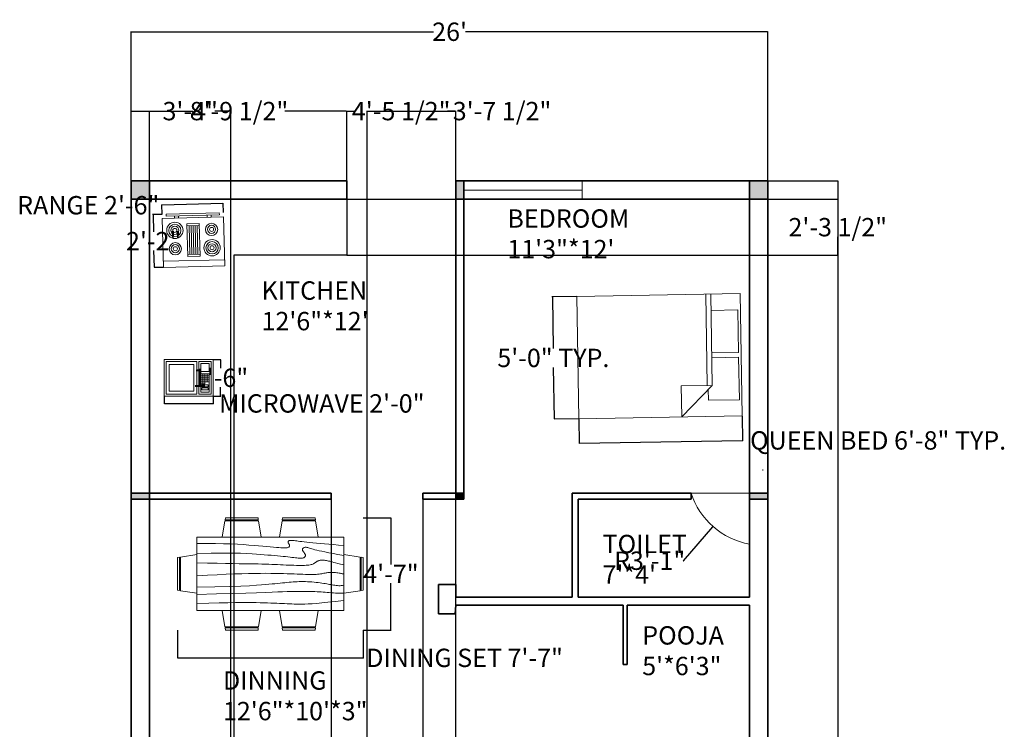
# Model space of a CAD drawing. Units: inches. Extents: x 23641 to 24129, y 27170 to 27889.
# Tile 2 of 2: x 23646 to 24129, y 27541 to 27889. Entities that reach past the tile are written whole.
import ezdxf

# ---------------------------------------------------------------- set-up
doc = ezdxf.new("R2010")
doc.units = ezdxf.units.IN
doc.header["$MEASUREMENT"] = 0
for name, color, linetype, lineweight in [('A-ANNO-DIMS', 2, 'Continuous', 18), ('A-AREA-IDEN', 7, 'Continuous', 25), ('A-DOOR', 4, 'Continuous', 18), ('A-EQPM', 9, 'Continuous', 18), ('A-FLOR-CASE', 8, 'Continuous', 25), ('A-FURN', 8, 'Continuous', 18), ('A-GLAZ', 4, 'Continuous', 18), ('A-WALL', 7, 'Continuous', 35), ('A-WALL-PATT', 7, 'Continuous', 13)]:
    doc.layers.add(name, color=color, linetype=linetype, lineweight=lineweight)
doc.styles.get("Standard").update_dxf_attribs({"font": 'arial.ttf'})
doc.dimstyles.get("Standard").update_dxf_attribs({"dimtxt": 9, "dimasz": 0.18, "dimexe": 0.18, "dimexo": 0.0625, "dimgap": 0.09, "dimtad": 0, "dimtih": 1, "dimtoh": 1, "dimdec": 0, "dimzin": 0, "dimdsep": 46, "dimlunit": 3, "dimtxsty": 'Standard', "dimcen": 0.09, "dimadec": 0, "dimazin": 0, "dimtfac": 1, "dimtdec": 0, "dimtofl": 0, "dimtmove": 0, "dimatfit": 3, "dimfxl": 1, "dimtolj": 1, "dimtzin": 0, "dimarcsym": 0})

# ---------------------------------------------------------------- blocks, each defined once
blk = doc.blocks.new('Range-Oven - 30 in top')
for p, q in [((0, -3), (30, -3)), ((12, -6), (18, -6)), ((13, -20), (13, -6)), ((14, -6), (14, -20)), ((15, -20), (15, -6)), ((16, -6), (16, -20)), ((17, -20), (17, -6)), ((6, -24), (6, -25)), ((8, -25), (8, -24)), ((18, -20), (12, -20)), ((22, -25), (22, -24)), ((24, -24), (24, -25))]:
    blk.add_line(p, q)
for points in [[(0, -24), (0, 0), (30, 0), (30, -24)], [(12, -21), (12, -5), (18, -5), (18, -21)], [(2, -26), (2, -25), (28, -25), (28, -26)]]:
    blk.add_lwpolyline(points, close=True)
for centre, radius in [((6, -9), 4), ((6, -9), 3), ((6, -9), 2), ((6, -9), 1), ((24, -9), 3), ((24, -9), 2), ((24, -9), 1), ((24, -18), 4), ((6, -18), 3), ((6, -18), 2), ((6, -18), 1), ((24, -18), 3), ((24, -18), 2), ((24, -18), 1)]:
    blk.add_circle(centre, radius)
blk = doc.blocks.new('Microwave')
for p, q in [((18, 10), (22, 10)), ((19, 7), (19, 11)), ((20, 11), (20, 7)), ((21, 7), (21, 11)), ((22, 9), (18, 9)), ((18, 8), (22, 8)), ((22, 7), (18, 7)), ((20, 6), (18, 6)), ((19, 6), (19, 7)), ((20, 7), (20, 6))]:
    blk.add_line(p, q)
for points in [[(0, 0), (0, 18), (24, 18), (24, 0)], [(1, 1), (1, 17), (16, 17), (16, 1)], [(2.5, 2.5), (2.5, 15.5), (14.5, 15.5), (14.5, 2.5)], [(17, 1), (17, 17), (23, 17), (23, 1)], [(18, 12), (18, 16), (22, 16), (22, 12)], [(18, 2), (18, 11), (22, 11), (22, 2)], [(18.5, 4.5), (18.5, 5.5), (21.5, 5.5), (21.5, 4.5)], [(18.5, 3), (18.5, 4), (21.5, 4), (21.5, 3)]]:
    blk.add_lwpolyline(points, close=True)
blk = doc.blocks.new('Dining Set - 36 x 72 in.')
for p, q in [((-22.2343, 26.00059), (-23.4847, 17.99762)), ((-22.2304, 26), (-5.7608, 26)), ((-22, 27.5), (-22.1562, 26.50042)), ((-5.8416, 26.5), (-22.1534, 26.5)), ((-22, 27.5), (-6, 27.5)), ((-5.8437, 26.49966), (-6, 27.5)), ((-4.5152, 17.99762), (-5.7655, 25.99926)), ((5.7657, 26.00059), (4.5153, 17.99762)), ((5.7696, 26), (22.2392, 26)), ((6, 27.5), (5.8438, 26.50042)), ((22.1584, 26.5), (5.8466, 26.5)), ((6, 27.5), (22, 27.5)), ((22.1563, 26.49966), (22, 27.5)), ((23.4848, 17.99762), (22.2345, 25.99926)), ((36, 18), (-36, 18)), ((-36, 18), (-36, -18)), ((36, -18), (36, 18)), ((-45.5, 8), (-44.5004, 8.15617)), ((-45.5, 8), (-45.5, -8)), ((-44.5, -8.15843), (-44.5, 8.15338)), ((-44.0006, 8.23428), (-35.9976, 9.48474)), ((-44, 8.23041), (-44, -8.23915)), ((44.0006, 8.23428), (35.9976, 9.48474)), ((44, 8.23041), (44, -8.23915)), ((44.5, -8.15843), (44.5, 8.15338)), ((45.5, 8), (44.5005, 8.15617)), ((45.5, 8), (45.5, -8)), ((-44.4997, -8.15631), (-45.5, -8)), ((-35.9976, -9.48476), (-43.9993, -8.2345)), ((35.9976, -9.48476), (43.9993, -8.2345)), ((44.4997, -8.15631), (45.5, -8)), ((-36, -18), (36, -18)), ((-22.2343, -26.0006), (-23.4847, -17.99762)), ((-4.5152, -17.99762), (-5.7655, -25.99928)), ((5.7657, -26.0006), (4.5153, -17.99762)), ((23.4848, -17.99762), (22.2345, -25.99928)), ((-22.2304, -26), (-5.7608, -26)), ((-22, -27.5), (-22.1562, -26.50044)), ((-5.8416, -26.5), (-22.1534, -26.5)), ((-22, -27.5), (-6, -27.5)), ((-5.8437, -26.49967), (-6, -27.5)), ((5.7696, -26), (22.2392, -26)), ((6, -27.5), (5.8438, -26.50044)), ((22.1584, -26.5), (5.8466, -26.5)), ((6, -27.5), (22, -27.5)), ((22.1563, -26.49967), (22, -27.5))]:
    blk.add_line(p, q)
for points in [[(-36, 15), (-31.1772, 14.97754), (-26.8079, 14.91406), (-22.8538, 14.81543), (-19.276, 14.6875), (-16.0362, 14.53613), (-13.0957, 14.36718), (-10.4159, 14.18652), (-7.9583, 14), (-5.6904, 13.81315), (-3.6035, 13.63021), (-1.6954, 13.45508), (0.0365, 13.29166), (1.5945, 13.14388), (2.9811, 13.01562), (4.1988, 12.9108), (5.25, 12.83333), (6.1393, 12.78613), (6.8802, 12.76823), (7.4883, 12.77767), (7.9792, 12.8125), (8.3685, 12.87077), (8.6719, 12.95052), (8.9049, 13.0498), (9.0833, 13.16666), (9.2205, 13.29899), (9.3216, 13.44401), (9.3895, 13.59879), (9.4271, 13.76041), (9.4373, 13.92594), (9.4232, 14.09245), (9.3875, 14.257), (9.3333, 14.41666), (9.2638, 14.56917), (9.1836, 14.71484), (9.0975, 14.85465), (9.0104, 14.98958), (8.9272, 15.1206), (8.8529, 15.2487), (8.7922, 15.37483), (8.75, 15.5), (8.7305, 15.62467), (8.7344, 15.74739), (8.7617, 15.86621), (8.8125, 15.97916), (8.8867, 16.08431), (8.9844, 16.17968), (9.1055, 16.26334), (9.25, 16.33333), (9.4189, 16.38802), (9.6172, 16.42708), (9.8506, 16.45052), (10.125, 16.45833), (10.4463, 16.45052), (10.8203, 16.42708), (11.2529, 16.38802), (11.75, 16.33333), (12.3184, 16.26318), (12.9694, 16.17838), (13.7151, 16.07991), (14.5677, 15.96875), (15.5395, 15.84586), (16.6426, 15.71224), (17.8893, 15.56884), (19.2917, 15.41666), (20.859, 15.25667), (22.5879, 15.08984), (24.4721, 14.91715), (26.5052, 14.73958), (28.6809, 14.5581), (30.9929, 14.3737), (33.4347, 14.18733), (36, 14)], [(-36, 10), (-28.9766, 10.14274), (-23.1725, 10.20442), (-18.4241, 10.19775), (-14.5677, 10.13541), (-11.4399, 10.03011), (-8.877, 9.89453), (-6.7154, 9.74137), (-4.7917, 9.58333), (-2.9698, 9.43082), (-1.2246, 9.28515), (0.4415, 9.14534), (2.026, 9.01041), (3.5266, 8.87939), (4.9408, 8.7513), (6.266, 8.62516), (7.5, 8.5), (8.6411, 8.37549), (9.6914, 8.2539), (10.6538, 8.13818), (11.5312, 8.03125), (12.3267, 7.93603), (13.043, 7.85547), (13.6831, 7.79248), (14.25, 7.75), (14.7471, 7.7303), (15.1797, 7.73307), (15.5537, 7.75732), (15.875, 7.80208), (16.1494, 7.86637), (16.3828, 7.94922), (16.5811, 8.04964), (16.75, 8.16666), (16.8944, 8.29915), (17.0143, 8.44531), (17.1089, 8.60319), (17.1771, 8.77083), (17.218, 8.94629), (17.2305, 9.1276), (17.2137, 9.31282), (17.1667, 9.5), (17.0895, 9.6875), (16.987, 9.875), (16.8649, 10.0625), (16.7292, 10.25), (16.5856, 10.4375), (16.4401, 10.625), (16.2985, 10.8125), (16.1667, 11), (16.05, 11.18733), (15.9518, 11.3737), (15.8752, 11.5581), (15.8229, 11.73958), (15.798, 11.91715), (15.8034, 12.08984), (15.842, 12.25667), (15.9167, 12.41666), (16.0295, 12.56836), (16.1784, 12.70833), (16.3605, 12.83268), (16.5729, 12.9375), (16.8127, 13.01888), (17.0768, 13.07291), (17.3625, 13.0957), (17.6667, 13.08333), (17.9894, 13.03312), (18.3418, 12.94726), (18.7382, 12.82918), (19.1927, 12.68229), (19.7195, 12.51001), (20.3327, 12.31575), (21.0465, 12.10294), (21.875, 11.875), (22.8357, 11.63354), (23.959, 11.37304), (25.2786, 11.08618), (26.8282, 10.76562), (28.6414, 10.40405), (30.752, 9.99414), (33.1936, 9.52856), (36, 9)], [(-36, 5.5), (-30.7157, 5.3348), (-26.069, 5.20963), (-21.9946, 5.11767), (-18.4271, 5.05208), (-15.3009, 5.00602), (-12.5508, 4.97265), (-10.1112, 4.94515), (-7.9167, 4.91666), (-5.909, 4.88167), (-4.0586, 4.83984), (-2.3429, 4.79215), (-0.7396, 4.73958), (0.7739, 4.6831), (2.22, 4.6237), (3.6213, 4.56233), (5, 4.5), (6.373, 4.43782), (7.7344, 4.3776), (9.0723, 4.32129), (10.375, 4.27083), (11.6309, 4.22819), (12.8281, 4.19531), (13.9551, 4.17415), (15, 4.16666), (15.954, 4.17448), (16.819, 4.19791), (17.6001, 4.23698), (18.3021, 4.29166), (18.9299, 4.36198), (19.4883, 4.44791), (19.9823, 4.54948), (20.4167, 4.66666), (20.7969, 4.79899), (21.1302, 4.94401), (21.4245, 5.09879), (21.6875, 5.26041), (21.9271, 5.42594), (22.1511, 5.59245), (22.3672, 5.757), (22.5834, 5.91666), (22.8065, 6.06868), (23.0404, 6.21093), (23.2879, 6.34147), (23.5521, 6.45833), (23.8358, 6.55957), (24.142, 6.64323), (24.4735, 6.70735), (24.8334, 6.75), (25.2235, 6.76969), (25.642, 6.76692), (26.0858, 6.74267), (26.5521, 6.69791), (27.0379, 6.63362), (27.5404, 6.55078), (28.0565, 6.45036), (28.5834, 6.33333), (29.1242, 6.19987), (29.7071, 6.04687), (30.3661, 5.87044), (31.1354, 5.66666), (32.0493, 5.43164), (33.142, 5.16146), (34.4475, 4.85221), (36, 4.5)], [(-36, -1), (-30.7915, -0.6591), (-26.0195, -0.38216), (-21.6519, -0.16284), (-17.6563, 0.00521), (-14.0005, 0.12833), (-10.6523, 0.21289), (-7.5796, 0.26522), (-4.75, 0.29166), (-2.134, 0.29793), (0.2878, 0.28711), (2.5317, 0.26163), (4.6146, 0.22396), (6.5529, 0.17651), (8.3633, 0.12174), (10.0623, 0.06209), (11.6667, 0), (13.1899, -0.06201), (14.6341, -0.1211), (15.9982, -0.17432), (17.2813, -0.21875), (18.4823, -0.25147), (19.6003, -0.26953), (20.6343, -0.27002), (21.5834, -0.25), (22.4481, -0.20768), (23.2357, -0.14584), (23.9549, -0.06836), (24.6146, 0.02083), (25.2235, 0.11784), (25.7904, 0.21875), (26.3241, 0.31966), (26.8334, 0.41666), (27.3265, 0.50618), (27.8099, 0.58593), (28.2894, 0.65397), (28.7709, 0.70833), (29.2601, 0.74707), (29.763, 0.76823), (30.2855, 0.76985), (30.8334, 0.75), (31.4088, 0.70784), (31.9994, 0.64713), (32.589, 0.57275), (33.1615, 0.48958), (33.7008, 0.4025), (34.1908, 0.3164), (34.6153, 0.23616), (34.9584, 0.16666), (35.2099, 0.11165), (35.3848, 0.07031), (35.504, 0.04069), (35.5886, 0.02083), (35.6594, 0.00879), (35.7377, 0.0026), (35.8442, 0.00032), (36, 0)], [(-36, -6.5), (-27.1843, -6.31267), (-20.084, -6.1263), (-14.469, -5.9419), (-10.1094, -5.76042), (-6.7752, -5.58285), (-4.2363, -5.41016), (-2.2629, -5.24333), (-0.625, -5.08334), (0.8708, -4.93099), (2.2715, -4.78646), (3.5872, -4.64974), (4.8281, -4.52084), (6.0046, -4.39974), (7.127, -4.28646), (8.2053, -4.18099), (9.25, -4.08334), (10.2705, -3.99382), (11.2734, -3.91407), (12.2647, -3.84603), (13.25, -3.79167), (14.2354, -3.75293), (15.2266, -3.73177), (16.2295, -3.73015), (17.25, -3.75), (18.2912, -3.79248), (19.3451, -3.85547), (20.4009, -3.93604), (21.4479, -4.03125), (22.4754, -4.13819), (23.4727, -4.25391), (24.4289, -4.37549), (25.3334, -4.5), (26.1785, -4.62492), (26.9694, -4.74935), (27.7145, -4.87281), (28.4219, -4.99479), (29.1, -5.11483), (29.7572, -5.23242), (30.4016, -5.34709), (31.0417, -5.45834), (31.6837, -5.56437), (32.3262, -5.65821), (32.9658, -5.73153), (33.599, -5.77604), (34.2224, -5.78345), (34.8327, -5.74545), (35.4264, -5.65373), (36, -5.5)], [(-36, -10), (-26.4022, -9.81299), (-18.4675, -9.62891), (-11.9839, -9.45069), (-6.7396, -9.28125), (-2.5226, -9.12354), (0.8789, -8.98047), (3.6769, -8.85498), (6.0833, -8.75), (8.2767, -8.66765), (10.3021, -8.60677), (12.1712, -8.56543), (13.8958, -8.54167), (15.4876, -8.53353), (16.9583, -8.53907), (18.3197, -8.55632), (19.5834, -8.58334), (20.7616, -8.61841), (21.8685, -8.66081), (22.9188, -8.71004), (23.9271, -8.76563), (24.9081, -8.82707), (25.8763, -8.89388), (26.8465, -8.96558), (27.8334, -9.04167), (28.8474, -9.12118), (29.8828, -9.20117), (30.93, -9.27824), (31.9792, -9.34896), (33.0205, -9.40991), (34.0443, -9.45768), (35.0407, -9.48885), (36, -9.5)], [(-36, -14.5), (-30.0881, -14.33513), (-25.0332, -14.21224), (-20.7312, -14.12647), (-17.0781, -14.07292), (-13.97, -14.04671), (-11.3027, -14.04297), (-8.9724, -14.05681), (-6.875, -14.08334), (-4.9224, -14.11833), (-3.0905, -14.16016), (-1.3709, -14.20785), (0.2448, -14.26042), (1.7647, -14.3169), (3.1973, -14.3763), (4.5507, -14.43767), (5.8333, -14.5), (7.0554, -14.5621), (8.235, -14.62175), (9.3922, -14.67652), (10.5469, -14.72396), (11.7192, -14.76164), (12.929, -14.78711), (14.1965, -14.79794), (15.5417, -14.79167), (16.9933, -14.76424), (18.6152, -14.70508), (20.4804, -14.60197), (22.6615, -14.44271), (25.2312, -14.21509), (28.2624, -13.9069), (31.8277, -13.50594), (36, -13)]]:
    blk.add_lwpolyline(points)
blk = doc.blocks.new('Bed - Queen')
for p, q in [((0, -80.00003), (0, 0)), ((0, 0), (59.99999, 0)), ((59.99999, 0), (59.99999, -80.00003)), ((7.99999, -1.2), (28.79998, -1.2)), ((7.99999, -14.4), (7.99999, -1.2)), ((28.79998, -1.2), (28.79998, -14.4)), ((31.19999, -1.2), (51.99999, -1.2)), ((31.19999, -14.4), (31.19999, -1.2)), ((51.99999, -1.2), (51.99999, -16.4)), ((0, -14.4), (44.8, -14.4)), ((59.99999, -29.6), (44.8, -14.4)), ((44.8, -14.4), (44.8, -29.6)), ((44.8, -16.8), (0, -16.8)), ((51.99999, -16.4), (46.79936, -16.4)), ((44.8, -29.6), (59.99999, -29.6)), ((59.99999, -80.00003), (0, -80.00003))]:
    blk.add_line(p, q)
blk = doc.blocks.new('*D10')
at = {"layer": 'A-ANNO-DIMS', "color": 0, "lineweight": -2, "transparency": 16777216}
for p, q in [((23700.98, 27810.33), (23700.98, 27883.62)), ((23701.16, 27883.44), (23849.18, 27883.44)), ((24012.8, 27883.44), (23864.79, 27883.44)), ((24012.98, 27810.33), (24012.98, 27883.62))]:
    blk.add_line(p, q, dxfattribs=at)
at = {"layer": 'A-ANNO-DIMS', "color": 0, "transparency": 16777216}
for points in [[(23701.16, 27883.47), (23701.16, 27883.41), (23700.98, 27883.44)], [(24012.8, 27883.47), (24012.8, 27883.41), (24012.98, 27883.44)]]:
    blk.add_solid(points, dxfattribs=at)
at = {"layer": 'Defpoints', "color": 0, "transparency": 16777216}
for p in [(24012.98, 27883.44), (23700.98, 27810.27), (24012.98, 27810.27)]:
    blk.add_point(p, dxfattribs=at)
at = {"layer": 'A-ANNO-DIMS', "color": 0, "transparency": 16777216, "insert": (23856.98, 27883.44), "char_height": 9, "attachment_point": 5}
blk.add_mtext("\\A1;26'", dxfattribs=at)
blk = doc.blocks.new('*D11')
at = {"layer": 'A-ANNO-DIMS', "color": 0, "lineweight": -2, "transparency": 16777216}
for p, q in [((23920.35, 27693.65), (23920.55, 27681.53)), ((24000.33, 27694.98), (24000.54, 27682.86)), ((23920.72, 27681.72), (24000.35, 27683.04)), ((24000.53, 27683.04), (24000.71, 27683.05))]:
    blk.add_line(p, q, dxfattribs=at)
at = {"layer": 'A-ANNO-DIMS', "color": 0, "transparency": 16777216}
for points in [[(23920.72, 27681.75), (23920.72, 27681.69), (23920.54, 27681.71)], [(24000.35, 27683.07), (24000.35, 27683.01), (24000.53, 27683.04)]]:
    blk.add_solid(points, dxfattribs=at)
at = {"layer": 'Defpoints', "color": 0, "transparency": 16777216}
for p in [(23920.34, 27693.71), (24000.33, 27695.04), (24000.53, 27683.04)]:
    blk.add_point(p, dxfattribs=at)
at = {"layer": 'A-ANNO-DIMS', "color": 0, "transparency": 16777216, "insert": (24067, 27683.05), "char_height": 9, "attachment_point": 5}
blk.add_mtext('\\A1;QUEEN BED 6\'-8" TYP.', dxfattribs=at)
blk = doc.blocks.new('*D12')
at = {"layer": 'A-ANNO-DIMS', "color": 0, "lineweight": -2, "transparency": 16777216}
for p, q in [((23919.29, 27753.7), (23907.17, 27753.5)), ((23907.35, 27753.32), (23907.77, 27728.19)), ((23908.34, 27693.69), (23907.93, 27718.82)), ((23920.28, 27693.71), (23908.17, 27693.51))]:
    blk.add_line(p, q, dxfattribs=at)
at = {"layer": 'A-ANNO-DIMS', "color": 0, "transparency": 16777216}
for points in [[(23907.38, 27753.32), (23907.32, 27753.32), (23907.35, 27753.5)], [(23908.37, 27693.69), (23908.31, 27693.69), (23908.35, 27693.51)]]:
    blk.add_solid(points, dxfattribs=at)
at = {"layer": 'Defpoints', "color": 0, "transparency": 16777216}
for p in [(23919.35, 27753.7), (23908.35, 27693.51), (23920.34, 27693.71)]:
    blk.add_point(p, dxfattribs=at)
at = {"layer": 'A-ANNO-DIMS', "color": 0, "transparency": 16777216, "insert": (23907.85, 27723.51), "char_height": 9, "attachment_point": 5}
blk.add_mtext('\\A1;5\'-0" TYP.', dxfattribs=at)
blk = doc.blocks.new('*D13')
at = {"layer": 'A-ANNO-DIMS', "color": 0, "lineweight": -2, "transparency": 16777216}
for p, q in [((23745.83, 27799.17), (23716.2, 27798.39)), ((23746.13, 27794.74), (23746, 27799.35)), ((23716.02, 27798.38), (23715.84, 27798.38)), ((23716.14, 27793.95), (23716.01, 27798.56))]:
    blk.add_line(p, q, dxfattribs=at)
at = {"layer": 'A-ANNO-DIMS', "color": 0, "transparency": 16777216}
for points in [[(23745.83, 27799.2), (23745.83, 27799.14), (23746.01, 27799.17)], [(23716.2, 27798.42), (23716.2, 27798.36), (23716.02, 27798.38)]]:
    blk.add_solid(points, dxfattribs=at)
at = {"layer": 'Defpoints', "color": 0, "transparency": 16777216}
for p in [(23716.02, 27798.38), (23746.13, 27794.68), (23716.14, 27793.88)]:
    blk.add_point(p, dxfattribs=at)
at = {"layer": 'A-ANNO-DIMS', "color": 0, "transparency": 16777216, "insert": (23679.92, 27798.38), "char_height": 9, "attachment_point": 5}
blk.add_mtext('\\A1;RANGE 2\'-6"', dxfattribs=at)
blk = doc.blocks.new('*D14')
at = {"layer": 'A-ANNO-DIMS', "color": 0, "lineweight": -2, "transparency": 16777216}
for p, q in [((23716.07, 27793.88), (23711.46, 27793.76)), ((23711.64, 27793.59), (23711.86, 27785.38)), ((23712.32, 27767.96), (23712.1, 27776.16)), ((23716.76, 27767.89), (23712.14, 27767.77))]:
    blk.add_line(p, q, dxfattribs=at)
at = {"layer": 'A-ANNO-DIMS', "color": 0, "transparency": 16777216}
for points in [[(23711.67, 27793.59), (23711.61, 27793.59), (23711.64, 27793.77)], [(23712.35, 27767.96), (23712.29, 27767.95), (23712.32, 27767.78)]]:
    blk.add_solid(points, dxfattribs=at)
at = {"layer": 'Defpoints', "color": 0, "transparency": 16777216}
for p in [(23716.14, 27793.88), (23712.32, 27767.78), (23716.82, 27767.89)]:
    blk.add_point(p, dxfattribs=at)
at = {"layer": 'A-ANNO-DIMS', "color": 0, "transparency": 16777216, "insert": (23711.98, 27780.77), "char_height": 9, "attachment_point": 5}
blk.add_mtext('\\A1;2\'-2"', dxfattribs=at)
blk = doc.blocks.new('*D15')
at = {"layer": 'A-ANNO-DIMS', "color": 0, "lineweight": -2, "transparency": 16777216}
for p, q in [((23717.12, 27704.71), (23717.12, 27701)), ((23741.12, 27704.71), (23741.12, 27701)), ((23717.3, 27701.18), (23740.94, 27701.18)), ((23741.12, 27701.18), (23741.3, 27701.18))]:
    blk.add_line(p, q, dxfattribs=at)
at = {"layer": 'A-ANNO-DIMS', "color": 0, "transparency": 16777216}
for points in [[(23717.3, 27701.21), (23717.3, 27701.15), (23717.12, 27701.18)], [(23740.94, 27701.21), (23740.94, 27701.15), (23741.12, 27701.18)]]:
    blk.add_solid(points, dxfattribs=at)
at = {"layer": 'Defpoints', "color": 0, "transparency": 16777216}
for p in [(23717.12, 27704.78), (23741.12, 27704.78), (23741.12, 27701.18)]:
    blk.add_point(p, dxfattribs=at)
at = {"layer": 'A-ANNO-DIMS', "color": 0, "transparency": 16777216, "insert": (23794.36, 27701.18), "char_height": 9, "attachment_point": 5}
blk.add_mtext('\\A1;MICROWAVE 2\'-0"', dxfattribs=at)
blk = doc.blocks.new('*D16')
at = {"layer": 'A-ANNO-DIMS', "color": 0, "lineweight": -2, "transparency": 16777216}
for p, q in [((23741.18, 27722.78), (23744.9, 27722.78)), ((23744.72, 27722.6), (23744.72, 27718.46)), ((23744.72, 27704.96), (23744.72, 27709.09)), ((23741.18, 27704.78), (23744.9, 27704.78))]:
    blk.add_line(p, q, dxfattribs=at)
at = {"layer": 'A-ANNO-DIMS', "color": 0, "transparency": 16777216}
for points in [[(23744.69, 27722.6), (23744.75, 27722.6), (23744.72, 27722.78)], [(23744.69, 27704.96), (23744.75, 27704.96), (23744.72, 27704.78)]]:
    blk.add_solid(points, dxfattribs=at)
at = {"layer": 'Defpoints', "color": 0, "transparency": 16777216}
for p in [(23741.12, 27722.78), (23744.72, 27722.78), (23741.12, 27704.78)]:
    blk.add_point(p, dxfattribs=at)
at = {"layer": 'A-ANNO-DIMS', "color": 0, "transparency": 16777216, "insert": (23744.72, 27713.78), "char_height": 9, "attachment_point": 5}
blk.add_mtext('\\A1;1\'-6"', dxfattribs=at)
blk = doc.blocks.new('*D21')
at = {"layer": 'A-ANNO-DIMS', "color": 0, "lineweight": -2, "transparency": 16777216}
for p, q in [((23723.6, 27590.02), (23723.6, 27576.26)), ((23814.6, 27590.02), (23814.6, 27576.26)), ((23723.78, 27576.44), (23814.42, 27576.44)), ((23814.6, 27576.44), (23814.78, 27576.44))]:
    blk.add_line(p, q, dxfattribs=at)
at = {"layer": 'A-ANNO-DIMS', "color": 0, "transparency": 16777216}
for points in [[(23723.78, 27576.47), (23723.78, 27576.41), (23723.6, 27576.44)], [(23814.42, 27576.47), (23814.42, 27576.41), (23814.6, 27576.44)]]:
    blk.add_solid(points, dxfattribs=at)
at = {"layer": 'Defpoints', "color": 0, "transparency": 16777216}
for p in [(23723.6, 27590.09), (23814.6, 27590.09), (23814.6, 27576.44)]:
    blk.add_point(p, dxfattribs=at)
at = {"layer": 'A-ANNO-DIMS', "color": 0, "transparency": 16777216, "insert": (23864.33, 27576.44), "char_height": 9, "attachment_point": 5}
blk.add_mtext('\\A1;DINING SET 7\'-7"', dxfattribs=at)
blk = doc.blocks.new('*D22')
at = {"layer": 'A-ANNO-DIMS', "color": 0, "lineweight": -2, "transparency": 16777216}
for p, q in [((23814.66, 27645.09), (23828.43, 27645.09)), ((23828.25, 27644.91), (23828.25, 27622.18)), ((23828.25, 27590.27), (23828.25, 27613)), ((23814.66, 27590.09), (23828.43, 27590.09))]:
    blk.add_line(p, q, dxfattribs=at)
at = {"layer": 'A-ANNO-DIMS', "color": 0, "transparency": 16777216}
for points in [[(23828.22, 27644.91), (23828.28, 27644.91), (23828.25, 27645.09)], [(23828.22, 27590.27), (23828.28, 27590.27), (23828.25, 27590.09)]]:
    blk.add_solid(points, dxfattribs=at)
at = {"layer": 'Defpoints', "color": 0, "transparency": 16777216}
for p in [(23814.6, 27645.09), (23828.25, 27645.09), (23814.6, 27590.09)]:
    blk.add_point(p, dxfattribs=at)
at = {"layer": 'A-ANNO-DIMS', "color": 0, "transparency": 16777216, "insert": (23828.25, 27617.59), "char_height": 9, "attachment_point": 5}
blk.add_mtext('\\A1;4\'-7"', dxfattribs=at)
blk = doc.blocks.new('*D23')
at = {"layer": 'A-ANNO-DIMS', "color": 0, "lineweight": -2, "transparency": 16777216}
for p, q in [((24013.05, 27810.27), (24047.41, 27810.27)), ((24047.23, 27810.09), (24047.23, 27514.96)), ((24047.23, 27210.45), (24047.23, 27505.59)), ((24013.05, 27210.27), (24047.41, 27210.27))]:
    blk.add_line(p, q, dxfattribs=at)
at = {"layer": 'A-ANNO-DIMS', "color": 0, "transparency": 16777216}
for points in [[(24047.2, 27810.09), (24047.26, 27810.09), (24047.23, 27810.27)], [(24047.2, 27210.45), (24047.26, 27210.45), (24047.23, 27210.27)]]:
    blk.add_solid(points, dxfattribs=at)
at = {"layer": 'Defpoints', "color": 0, "transparency": 16777216}
for p in [(24012.98, 27810.27), (24047.23, 27810.27), (24012.98, 27210.27)]:
    blk.add_point(p, dxfattribs=at)
at = {"layer": 'A-ANNO-DIMS', "color": 0, "transparency": 16777216, "insert": (24047.23, 27510.27), "char_height": 9, "attachment_point": 5}
blk.add_mtext('\\A1;50\'-0"', dxfattribs=at)
blk = doc.blocks.new('*D24')
at = {"layer": 'A-ANNO-DIMS', "color": 0, "lineweight": -2, "transparency": 16777216}
for p, q in [((23806.55, 27810.33), (23806.55, 27844.7)), ((23806.73, 27844.52), (23810.55, 27844.52)), ((23859.8, 27844.52), (23855.99, 27844.52)), ((23859.98, 27810.33), (23859.98, 27844.7))]:
    blk.add_line(p, q, dxfattribs=at)
at = {"layer": 'A-ANNO-DIMS', "color": 0, "transparency": 16777216}
for points in [[(23806.73, 27844.55), (23806.73, 27844.49), (23806.55, 27844.52)], [(23859.8, 27844.55), (23859.8, 27844.49), (23859.98, 27844.52)]]:
    blk.add_solid(points, dxfattribs=at)
at = {"layer": 'Defpoints', "color": 0, "transparency": 16777216}
for p in [(23859.98, 27844.52), (23806.55, 27810.27), (23859.98, 27810.27)]:
    blk.add_point(p, dxfattribs=at)
at = {"layer": 'A-ANNO-DIMS', "color": 0, "transparency": 16777216, "insert": (23833.27, 27844.52), "char_height": 9, "attachment_point": 5}
blk.add_mtext('\\A1;4\'-5 1/2"', dxfattribs=at)
blk = doc.blocks.new('*D25')
at = {"layer": 'A-ANNO-DIMS', "color": 0, "lineweight": -2, "transparency": 16777216}
for p, q in [((23709.98, 27315.33), (23709.98, 27844.7)), ((23710.16, 27844.52), (23717.83, 27844.52)), ((23749.6, 27844.52), (23741.93, 27844.52)), ((23749.78, 27315.33), (23749.78, 27844.7))]:
    blk.add_line(p, q, dxfattribs=at)
at = {"layer": 'A-ANNO-DIMS', "color": 0, "transparency": 16777216}
for points in [[(23710.16, 27844.55), (23710.16, 27844.49), (23709.98, 27844.52)], [(23749.6, 27844.55), (23749.6, 27844.49), (23749.78, 27844.52)]]:
    blk.add_solid(points, dxfattribs=at)
at = {"layer": 'Defpoints', "color": 0, "transparency": 16777216}
for p in [(23749.78, 27844.52), (23709.98, 27315.27), (23749.78, 27315.27)]:
    blk.add_point(p, dxfattribs=at)
at = {"layer": 'A-ANNO-DIMS', "color": 0, "transparency": 16777216, "insert": (23729.88, 27844.52), "char_height": 9, "attachment_point": 5}
blk.add_mtext('\\A1;3\'-4"', dxfattribs=at)
blk = doc.blocks.new('*D28')
at = {"layer": 'A-ANNO-DIMS', "color": 0, "lineweight": -2, "transparency": 16777216}
for p, q in [((23700.98, 27810.33), (23700.98, 27844.7)), ((23701.16, 27844.52), (23731.22, 27844.52)), ((23806.37, 27844.52), (23776.31, 27844.52)), ((23806.55, 27810.33), (23806.55, 27844.7))]:
    blk.add_line(p, q, dxfattribs=at)
at = {"layer": 'A-ANNO-DIMS', "color": 0, "transparency": 16777216}
for points in [[(23701.16, 27844.55), (23701.16, 27844.49), (23700.98, 27844.52)], [(23806.37, 27844.55), (23806.37, 27844.49), (23806.55, 27844.52)]]:
    blk.add_solid(points, dxfattribs=at)
at = {"layer": 'Defpoints', "color": 0, "transparency": 16777216}
for p in [(23806.55, 27844.52), (23700.98, 27810.27), (23806.55, 27810.27)]:
    blk.add_point(p, dxfattribs=at)
at = {"layer": 'A-ANNO-DIMS', "color": 0, "transparency": 16777216, "insert": (23753.77, 27844.52), "char_height": 9, "attachment_point": 5}
blk.add_mtext('\\A1;8\'-9 1/2"', dxfattribs=at)
blk = doc.blocks.new('*D29')
at = {"layer": 'A-ANNO-DIMS', "color": 0, "lineweight": -2, "transparency": 16777216}
for p, q in [((23799.02, 27654.21), (23799.02, 27175.84)), ((23843.92, 27654.21), (23843.92, 27175.84)), ((23799.2, 27176.02), (23809.42, 27176.02)), ((23843.74, 27176.02), (23833.52, 27176.02))]:
    blk.add_line(p, q, dxfattribs=at)
at = {"layer": 'A-ANNO-DIMS', "color": 0, "transparency": 16777216}
for points in [[(23799.2, 27176.05), (23799.2, 27175.99), (23799.02, 27176.02)], [(23843.74, 27176.05), (23843.74, 27175.99), (23843.92, 27176.02)]]:
    blk.add_solid(points, dxfattribs=at)
at = {"layer": 'Defpoints', "color": 0, "transparency": 16777216}
for p in [(23799.02, 27654.27), (23843.92, 27654.27), (23843.92, 27176.02)]:
    blk.add_point(p, dxfattribs=at)
at = {"layer": 'A-ANNO-DIMS', "color": 0, "transparency": 16777216, "insert": (23821.47, 27176.02), "char_height": 9, "attachment_point": 5}
blk.add_mtext('\\A1;3\'-9"', dxfattribs=at)
blk = doc.blocks.new('*D30')
at = {"layer": 'A-ANNO-DIMS', "color": 0, "lineweight": -2, "transparency": 16777216}
for p, q in [((23709.98, 27657.21), (23709.98, 27175.84)), ((23751.17, 27657.21), (23751.17, 27175.84)), ((23710.16, 27176.02), (23718.53, 27176.02)), ((23750.99, 27176.02), (23742.63, 27176.02))]:
    blk.add_line(p, q, dxfattribs=at)
at = {"layer": 'A-ANNO-DIMS', "color": 0, "transparency": 16777216}
for points in [[(23710.16, 27176.05), (23710.16, 27175.99), (23709.98, 27176.02)], [(23750.99, 27176.05), (23750.99, 27175.99), (23751.17, 27176.02)]]:
    blk.add_solid(points, dxfattribs=at)
at = {"layer": 'Defpoints', "color": 0, "transparency": 16777216}
for p in [(23709.98, 27657.27), (23751.17, 27657.27), (23751.17, 27176.02)]:
    blk.add_point(p, dxfattribs=at)
at = {"layer": 'A-ANNO-DIMS', "color": 0, "transparency": 16777216, "insert": (23730.58, 27176.02), "char_height": 9, "attachment_point": 5}
blk.add_mtext('\\A1;3\'-5"', dxfattribs=at)
blk = doc.blocks.new('*D31')
at = {"layer": 'A-ANNO-DIMS', "color": 0, "lineweight": -2, "transparency": 16777216}
for p, q in [((23806.61, 27801.27), (24047.41, 27801.27)), ((24047.23, 27801.09), (24047.23, 27792.36)), ((24047.23, 27774.14), (24047.23, 27782.87)), ((23806.61, 27773.96), (24047.41, 27773.96))]:
    blk.add_line(p, q, dxfattribs=at)
at = {"layer": 'A-ANNO-DIMS', "color": 0, "transparency": 16777216}
for points in [[(24047.2, 27801.09), (24047.26, 27801.09), (24047.23, 27801.27)], [(24047.2, 27774.14), (24047.26, 27774.14), (24047.23, 27773.96)]]:
    blk.add_solid(points, dxfattribs=at)
at = {"layer": 'Defpoints', "color": 0, "transparency": 16777216}
for p in [(23806.55, 27801.27), (23806.55, 27773.96), (24047.23, 27773.96)]:
    blk.add_point(p, dxfattribs=at)
at = {"layer": 'A-ANNO-DIMS', "color": 0, "transparency": 16777216, "insert": (24047.23, 27787.61), "char_height": 9, "attachment_point": 5}
blk.add_mtext('\\A1;2\'-3 1/2"', dxfattribs=at)
blk = doc.blocks.new('*D35')
at = {"layer": 'A-ANNO-DIMS', "color": 0, "lineweight": -2, "transparency": 16777216}
for p, q in [((23816.62, 27531.33), (23816.62, 27844.7)), ((23816.8, 27844.52), (23859.8, 27844.52)), ((23859.98, 27531.33), (23859.98, 27844.7)), ((23859.98, 27844.52), (23860.16, 27844.52))]:
    blk.add_line(p, q, dxfattribs=at)
at = {"layer": 'A-ANNO-DIMS', "color": 0, "transparency": 16777216}
for points in [[(23816.8, 27844.55), (23816.8, 27844.49), (23816.62, 27844.52)], [(23859.8, 27844.55), (23859.8, 27844.49), (23859.98, 27844.52)]]:
    blk.add_solid(points, dxfattribs=at)
at = {"layer": 'Defpoints', "color": 0, "transparency": 16777216}
for p in [(23859.98, 27844.52), (23816.62, 27531.27), (23859.98, 27531.27)]:
    blk.add_point(p, dxfattribs=at)
at = {"layer": 'A-ANNO-DIMS', "color": 0, "transparency": 16777216, "insert": (23882.7, 27844.52), "char_height": 9, "attachment_point": 5}
blk.add_mtext('\\A1;3\'-7 1/2"', dxfattribs=at)
blk = doc.blocks.new('*D38')
at = {"layer": 'A-ANNO-DIMS', "color": 0, "lineweight": -2, "transparency": 16777216}
for p, q in [((24010.43, 27668.62), (24010.61, 27668.62)), ((24010.52, 27668.53), (24010.52, 27668.71)), ((23971.58, 27624.07), (23986.07, 27640.64)), ((23971.4, 27624.07), (23971.58, 27624.07))]:
    blk.add_line(p, q, dxfattribs=at)
at = {"layer": 'A-ANNO-DIMS', "color": 0, "transparency": 16777216}
blk.add_solid([(23986.04, 27640.66), (23986.09, 27640.62), (23986.18, 27640.78)], dxfattribs=at)
at = {"layer": 'Defpoints', "color": 0, "transparency": 16777216}
for p in [(24010.52, 27668.62), (23986.18, 27640.78)]:
    blk.add_point(p, dxfattribs=at)
at = {"layer": 'A-ANNO-DIMS', "color": 0, "transparency": 16777216, "insert": (23955.04, 27624.07), "char_height": 9, "attachment_point": 5}
blk.add_mtext('\\A1;R3\'-1"', dxfattribs=at)

msp = doc.modelspace()

# ---------------------------------------------------------------- hatches: boundary and pattern name
at = {"layer": 'A-WALL-PATT'}
h = msp.add_hatch(color=256, dxfattribs=at)
h.dxf.hatch_style = 1
h.paths.add_polyline_path([(23709.98, 27810.27), (23700.98, 27810.27), (23700.98, 27801.27), (23709.98, 27801.27)])
h = msp.add_hatch(color=256, dxfattribs=at)
h.dxf.hatch_style = 1
h.paths.add_polyline_path([(23863.98, 27810.27), (23859.98, 27810.27), (23859.98, 27801.27), (23863.98, 27801.27)])
h = msp.add_hatch(color=256, dxfattribs=at)
h.dxf.hatch_style = 1
h.paths.add_polyline_path([(24012.98, 27810.27), (24003.98, 27810.27), (24003.98, 27801.27), (24012.98, 27801.27)])
h = msp.add_hatch(color=256, dxfattribs=at)
h.dxf.hatch_style = 1
h.paths.add_polyline_path([(23709.98, 27657.27), (23700.98, 27657.27), (23700.98, 27654.27), (23709.98, 27654.27)])
h = msp.add_hatch(color=256, dxfattribs=at)
h.dxf.hatch_style = 1
h.paths.add_polyline_path([(23863.98, 27657.27), (23859.98, 27657.27), (23859.98, 27654.27), (23863.98, 27654.27)])
h = msp.add_hatch(color=256, dxfattribs=at)
h.dxf.hatch_style = 1
h.paths.add_polyline_path([(23863.98, 27657.27), (23859.98, 27657.27), (23859.98, 27654.27), (23863.98, 27654.27)])
h = msp.add_hatch(color=256, dxfattribs=at)
h.dxf.hatch_style = 1
h.paths.add_polyline_path([(24012.98, 27657.27), (24003.98, 27657.27), (24003.98, 27654.27), (24012.98, 27654.27)])

# ---------------------------------------------------------------- linework, layer by layer
at = {"layer": 'A-DOOR'}
msp.add_line((23975.33, 27657.27), (24003.98, 27657.27), dxfattribs=at)
msp.add_arc((24010.52, 27668.62), 36.98, 197.8747, 259.8178, dxfattribs=at)
at = {"layer": 'A-FLOR-CASE'}
for p, q in [((23806.55, 27801.27), (23806.55, 27773.96)), ((23806.55, 27773.96), (23751.17, 27773.96)), ((23751.17, 27773.96), (23751.17, 27657.27))]:
    msp.add_line(p, q, dxfattribs=at)
at = {"layer": 'A-GLAZ'}
for p, q in [((23921.91, 27810.27), (23921.91, 27801.27)), ((23863.98, 27805.77), (23921.91, 27805.77)), ((23863.98, 27801.27), (23916.98, 27801.27))]:
    msp.add_line(p, q, dxfattribs=at)
at = {"layer": 'A-WALL'}
for p, q in [((23709.98, 27801.27), (23709.98, 27810.27)), ((23806.55, 27810.27), (23806.55, 27801.27)), ((23859.98, 27801.27), (23859.98, 27810.27)), ((23863.98, 27801.27), (23863.98, 27810.27)), ((24003.98, 27801.27), (24003.98, 27810.27)), ((23709.98, 27801.27), (23700.98, 27801.27)), ((23709.98, 27801.27), (23806.55, 27801.27)), ((23709.98, 27657.27), (23709.98, 27801.27)), ((23859.98, 27657.27), (23859.98, 27801.27)), ((23863.98, 27801.27), (23859.98, 27801.27)), ((23863.98, 27657.27), (23863.98, 27801.27)), ((23863.98, 27801.27), (24003.98, 27801.27)), ((24003.98, 27801.27), (24003.98, 27657.27)), ((24003.98, 27801.27), (24012.98, 27801.27)), ((23709.98, 27657.27), (23700.98, 27657.27)), ((23709.98, 27657.27), (23799.02, 27657.27)), ((23709.98, 27654.27), (23709.98, 27657.27)), ((23799.02, 27657.27), (23799.02, 27654.27)), ((23843.92, 27654.27), (23843.92, 27657.27)), ((23843.92, 27657.27), (23859.98, 27657.27)), ((23859.98, 27657.27), (23863.98, 27657.27)), ((23859.98, 27657.27), (23859.98, 27654.27)), ((23863.98, 27657.27), (23863.98, 27654.27)), ((23916.98, 27657.27), (23916.98, 27606.27)), ((23916.98, 27657.27), (23975.33, 27657.27)), ((23975.33, 27657.27), (23975.33, 27654.27)), ((24003.98, 27657.27), (24003.98, 27654.27)), ((24003.98, 27657.27), (24012.98, 27657.27)), ((23709.98, 27654.27), (23700.98, 27654.27)), ((23709.98, 27654.27), (23799.02, 27654.27)), ((23709.98, 27531.27), (23709.98, 27654.27)), ((23859.98, 27654.27), (23843.92, 27654.27)), ((23859.98, 27654.27), (23863.98, 27654.27)), ((23919.98, 27654.27), (23919.98, 27606.27)), ((23919.98, 27654.27), (23975.33, 27654.27)), ((24003.98, 27654.27), (24003.98, 27606.27)), ((24003.98, 27654.27), (24012.98, 27654.27)), ((23859.98, 27612.43), (23851.51, 27612.43)), ((23851.51, 27612.43), (23851.51, 27597.98)), ((23859.98, 27606.27), (23859.98, 27612.43)), ((23859.98, 27606.27), (23916.98, 27606.27)), ((23919.98, 27606.27), (24003.98, 27606.27)), ((23859.69, 27597.98), (23859.98, 27602.27)), ((23859.98, 27602.27), (23941.98, 27602.27)), ((23941.98, 27602.27), (23941.98, 27573.25)), ((23943.98, 27602.27), (23943.98, 27573.25)), ((23943.98, 27602.27), (24003.98, 27602.27)), ((24003.98, 27602.27), (24003.98, 27527.27)), ((23851.51, 27597.98), (23859.69, 27597.98)), ((23941.98, 27573.25), (23943.98, 27573.25))]:
    msp.add_line(p, q, dxfattribs=at)
msp.add_lwpolyline([(23859.98, 27810.27), (24012.98, 27810.27), (24012.98, 27210.27), (23700.98, 27210.27), (23700.98, 27810.27), (23806.55, 27810.27)], dxfattribs=at)

# ---------------------------------------------------------------- block references
at = {"layer": 'A-EQPM', "rotation": 181.5092603108288}
msp.add_blockref('Range-Oven - 30 in top', (23746.81, 27768.68), dxfattribs=at)
at = {"layer": 'A-EQPM'}
msp.add_blockref('Microwave', (23717.12, 27704.78), dxfattribs=at)
at = {"layer": 'A-FURN', "rotation": 270.9522082565971}
msp.add_blockref('Bed - Queen', (23999.34, 27755.03), dxfattribs=at)
at = {"layer": 'A-FURN'}
msp.add_blockref('Dining Set - 36 x 72 in.', (23769.1, 27617.59), dxfattribs=at)

# ---------------------------------------------------------------- texts
at = {"layer": 'A-AREA-IDEN', "char_height": 9, "attachment_point": 1}
for s, insert in [('BEDROOM\\P11\'3"*12\'', (23885.31, 27796.36)), ('KITCHEN\\P12\'6"*12\'', (23764.84, 27761.06)), ("TOILET\\P7'*4'", (23931.96, 27636.78)), ('POOJA\\P5\'*6\'3"', (23951.4, 27591.96)), ('DINNING\\P12\'6"*10\'*3"', (23745.93, 27569.85))]:
    msp.add_mtext_dynamic_manual_height_columns(s, width=25.8959, gutter_width=1, heights=[0], dxfattribs=dict(at, insert=insert))

# ---------------------------------------------------------------- dimensions: what is measured, and where the dimension line sits
at = {"layer": 'A-ANNO-DIMS'}
for base, p1, p2, override, picture, middle in [((24012.98, 27883.44), (23700.98, 27810.27), (24012.98, 27810.27), {"dimclrd": 0, "dimclre": 0, "dimclrt": 0}, '*D10', (23856.98, 27883.44)), ((23806.55, 27844.52), (23700.98, 27810.27), (23806.55, 27810.27), {"dimdec": 1, "dimlfac": 1, "dimrnd": 0, "dimzin": 1, "dimdsep": 46, "dimlunit": 4, "dimfrac": 2}, '*D28', (23753.77, 27844.52)), ((23859.98, 27844.52), (23806.55, 27810.27), (23859.98, 27810.27), {"dimdec": 1, "dimlfac": 1, "dimrnd": 0, "dimzin": 1, "dimdsep": 46, "dimlunit": 4, "dimfrac": 2}, '*D24', (23833.27, 27844.52)), ((23859.98, 27844.52), (23816.62, 27531.27), (23859.98, 27531.27), {"dimdec": 1, "dimlfac": 1, "dimrnd": 0, "dimzin": 1, "dimdsep": 46, "dimlunit": 4, "dimfrac": 2}, '*D35', (23882.7, 27844.52)), ((23749.78, 27844.52), (23709.98, 27315.27), (23749.78, 27315.27), {"dimdec": 1, "dimlfac": 1, "dimrnd": 0, "dimzin": 1, "dimdsep": 46, "dimlunit": 4, "dimfrac": 2}, '*D25', (23729.88, 27844.52)), ((23751.17, 27176.02), (23709.98, 27657.27), (23751.17, 27657.27), {"dimdec": 1, "dimlfac": 1, "dimrnd": 0, "dimzin": 1, "dimdsep": 46, "dimlunit": 4, "dimfrac": 2}, '*D30', (23730.58, 27176.02)), ((23843.92, 27176.02), (23799.02, 27654.27), (23843.92, 27654.27), {"dimdec": 1, "dimlfac": 1, "dimrnd": 0, "dimzin": 1, "dimdsep": 46, "dimlunit": 4, "dimfrac": 2}, '*D29', (23821.47, 27176.02))]:
    dim = msp.add_linear_dim(base=base, p1=p1, p2=p2, dimstyle='Standard', override=override, dxfattribs=at)
    dim.commit()
    dim.dimension.update_dxf_attribs({"geometry": picture, "text_midpoint": middle})
for base, p1, p2, angle, text, picture, middle in [((23716.02, 27798.38), (23746.13, 27794.68), (23716.14, 27793.88), 181.5093, 'RANGE <>', '*D13', (23679.92, 27798.38)), ((23908.35, 27693.51), (23919.35, 27753.7), (23920.34, 27693.71), 270.9522, '<> TYP.', '*D12', (23907.85, 27723.51)), ((24000.53, 27683.04), (23920.34, 27693.71), (24000.33, 27695.04), 0.9522, 'QUEEN BED <> TYP.', '*D11', (24067, 27683.05))]:
    dim = msp.add_linear_dim(base=base, p1=p1, p2=p2, angle=angle, text=text, dimstyle='Standard', override={"dimdec": 1, "dimlfac": 1, "dimrnd": 0, "dimzin": 1, "dimdsep": 46, "dimlunit": 4, "dimfrac": 2}, dxfattribs=at)
    dim.commit()
    dim.dimension.update_dxf_attribs({"geometry": picture, "text_midpoint": middle})
for base, p1, p2, angle, picture, middle in [((24047.23, 27810.27), (24012.98, 27210.27), (24012.98, 27810.27), 90, '*D23', (24047.23, 27510.27)), ((24047.23, 27773.96), (23806.55, 27801.27), (23806.55, 27773.96), 90, '*D31', (24047.23, 27787.61)), ((23712.32, 27767.78), (23716.14, 27793.88), (23716.82, 27767.89), 271.5093, '*D14', (23711.98, 27780.77)), ((23744.72, 27722.78), (23741.12, 27704.78), (23741.12, 27722.78), 90, '*D16', (23744.72, 27713.78)), ((23828.25, 27645.09), (23814.6, 27590.09), (23814.6, 27645.09), 90, '*D22', (23828.25, 27617.59))]:
    dim = msp.add_linear_dim(base=base, p1=p1, p2=p2, angle=angle, dimstyle='Standard', override={"dimdec": 1, "dimlfac": 1, "dimrnd": 0, "dimzin": 1, "dimdsep": 46, "dimlunit": 4, "dimfrac": 2}, dxfattribs=at)
    dim.commit()
    dim.dimension.update_dxf_attribs({"geometry": picture, "text_midpoint": middle})
for base, p1, p2, text, picture, middle in [((23741.12, 27701.18), (23717.12, 27704.78), (23741.12, 27704.78), 'MICROWAVE <>', '*D15', (23794.36, 27701.18)), ((23814.6, 27576.44), (23723.6, 27590.09), (23814.6, 27590.09), 'DINING SET <>', '*D21', (23864.33, 27576.44))]:
    dim = msp.add_linear_dim(base=base, p1=p1, p2=p2, text=text, dimstyle='Standard', override={"dimdec": 1, "dimlfac": 1, "dimrnd": 0, "dimzin": 1, "dimdsep": 46, "dimlunit": 4, "dimfrac": 2}, dxfattribs=at)
    dim.commit()
    dim.dimension.update_dxf_attribs({"geometry": picture, "text_midpoint": middle})
dim = msp.add_radius_dim(center=(24010.52, 27668.62), mpoint=(23986.18, 27640.78), dimstyle='Standard', override={"dimdec": 1, "dimlfac": 1, "dimrnd": 0, "dimzin": 1, "dimdsep": 46, "dimlunit": 4, "dimfrac": 2}, dxfattribs=at)
dim.commit()
dim.dimension.update_dxf_attribs({"geometry": '*D38', "text_midpoint": (23955.04, 27624.07), "dimtype": 164})

doc.saveas('drawing.dxf')
